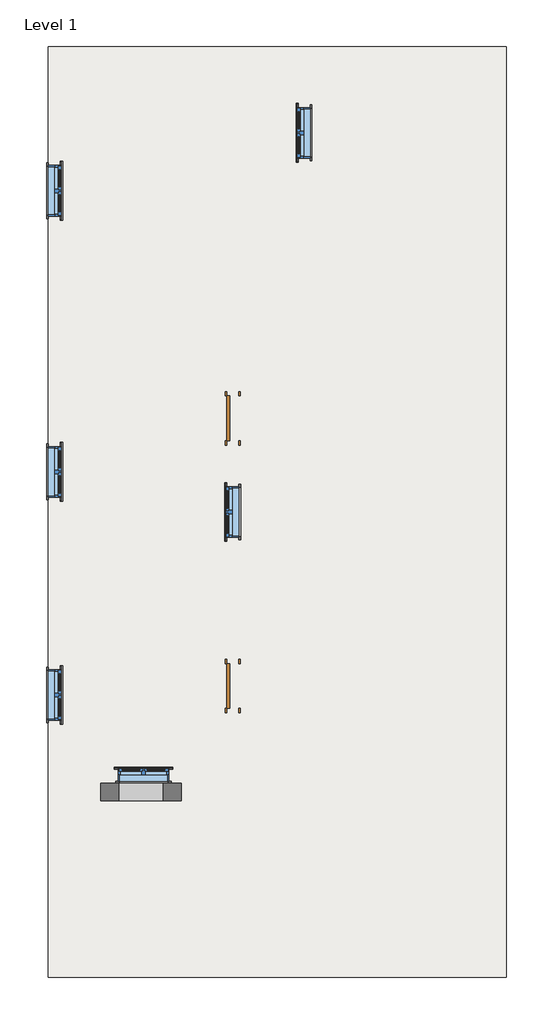
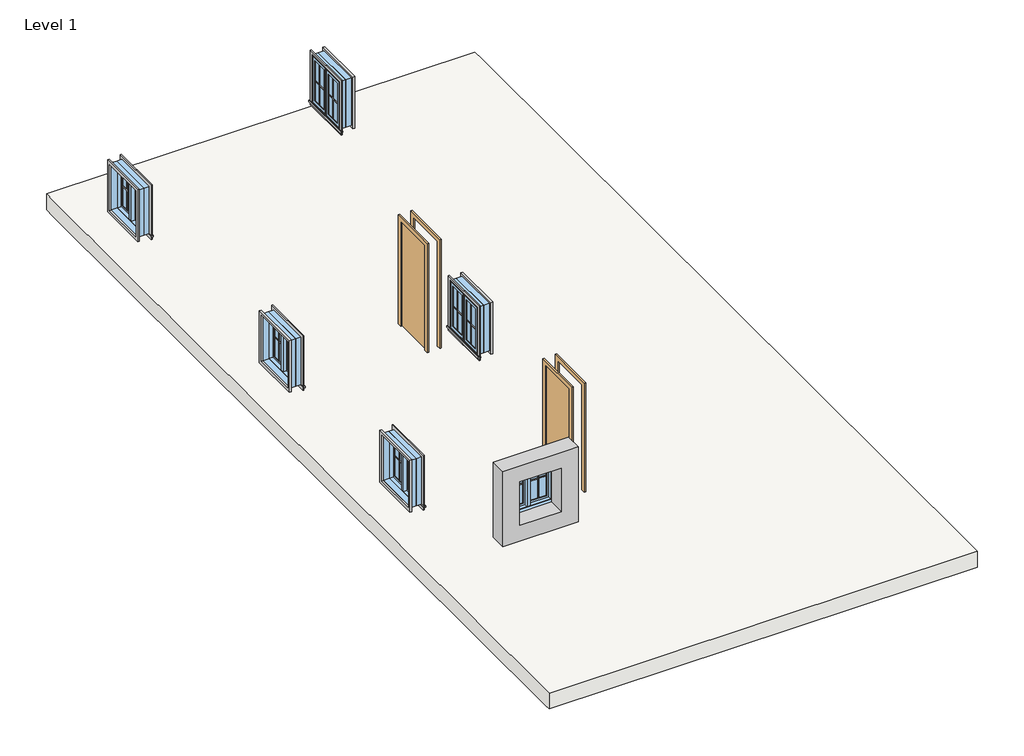
# One storey: 24 proxies, 6 windows, 2 doors, 1 air terminal, 1 slab.
"""IFC4 building model written with IfcOpenShell, lengths in millimetres."""

from ifc_helpers import new_model, si_unit, origin, place, context, project, spatial, faceted_brep, transform, mapped, element, save
from components import air_terminals_1_air_terminals_1_01c5ecaf, muntin_pattern_2x2_muntin_pattern_2x2_b3fe6957, muntin_pattern_2x2_muntin_pattern_2x2_3e0ecaf2, trim_window_exterior_flat_with_sill_41619996, trim_window_interior_flat_picture_frame_51c85655, door_fadea3f2, window_c29befe5

model = new_model("IFC4")

# Units and contexts
model_context = context("Model", 3, world=origin())
ifc_project = project(units=[si_unit("LENGTHUNIT", "METRE", prefix="MILLI")], contexts=[model_context])

# Site, building, storey
site = spatial("IfcSite", under=ifc_project)
building = spatial("IfcBuilding", under=site)
storey = spatial("IfcBuildingStorey", under=building, Name="Level 1", Elevation=5486.4)

# Air terminal
placement = place(None, origin())
air_terminals_1_air_terminals_1_shape = air_terminals_1_air_terminals_1_01c5ecaf(model_context)
element("IfcAirTerminal", 1, ObjectType="Air Terminals 1 : Air Terminals 1", at=placement, inside=storey, context=model_context, shape_type="MappedRepresentation", body=[
    mapped(air_terminals_1_air_terminals_1_shape, transform((0.0, 0.0, 0.0), x_axis=(1.0, 0.0, 0.0), y_axis=(0.0, 1.0, 0.0), z_axis=(0.0, 0.0, 1.0))),
])

# Proxies
muntin_pattern_2x2_muntin_pattern_2x2_shape = muntin_pattern_2x2_muntin_pattern_2x2_b3fe6957(model_context)
element("IfcBuildingElementProxy", 2, Name="Muntin Pattern_2x2 : Muntin Pattern_2x2", ObjectType="Muntin Pattern_2x2 : Muntin Pattern_2x2", at=placement, inside=storey, context=model_context, shape_type="MappedRepresentation", body=[
    mapped(muntin_pattern_2x2_muntin_pattern_2x2_shape, transform((-14472.8012549, 3709.9777962, 6470.65), x_axis=(1.0, 0.0, 0.0), y_axis=(0.0, 1.0, 0.0), z_axis=(0.0, 0.0, 1.0))),
])
element("IfcBuildingElementProxy", 3, Name="Muntin Pattern_2x2 : Muntin Pattern_2x2", ObjectType="Muntin Pattern_2x2 : Muntin Pattern_2x2", at=placement, inside=storey, context=model_context, shape_type="MappedRepresentation", body=[
    mapped(muntin_pattern_2x2_muntin_pattern_2x2_shape, transform((-12826.5637549, 7899.3902962, 6470.65), x_axis=(0.0, 1.0, 0.0), y_axis=(-1.0, 0.0, 0.0), z_axis=(0.0, 0.0, 1.0))),
])
element("IfcBuildingElementProxy", 4, Name="Muntin Pattern_2x2 : Muntin Pattern_2x2", ObjectType="Muntin Pattern_2x2 : Muntin Pattern_2x2", at=placement, inside=storey, context=model_context, shape_type="MappedRepresentation", body=[
    mapped(muntin_pattern_2x2_muntin_pattern_2x2_shape, transform((-15690.4137549, 13814.4152962, 6470.65), x_axis=(0.0, -1.0, 0.0), y_axis=(1.0, 0.0, 0.0), z_axis=(0.0, 0.0, 1.0))),
])
element("IfcBuildingElementProxy", 5, Name="Muntin Pattern_2x2 : Muntin Pattern_2x2", ObjectType="Muntin Pattern_2x2 : Muntin Pattern_2x2", at=placement, inside=storey, context=model_context, shape_type="MappedRepresentation", body=[
    mapped(muntin_pattern_2x2_muntin_pattern_2x2_shape, transform((-15690.4137549, 9013.8152962, 6470.65), x_axis=(0.0, -1.0, 0.0), y_axis=(1.0, 0.0, 0.0), z_axis=(0.0, 0.0, 1.0))),
])
element("IfcBuildingElementProxy", 6, Name="Muntin Pattern_2x2 : Muntin Pattern_2x2", ObjectType="Muntin Pattern_2x2 : Muntin Pattern_2x2", at=placement, inside=storey, context=model_context, shape_type="MappedRepresentation", body=[
    mapped(muntin_pattern_2x2_muntin_pattern_2x2_shape, transform((-15690.4137549, 5203.8152962, 6470.65), x_axis=(0.0, -1.0, 0.0), y_axis=(1.0, 0.0, 0.0), z_axis=(0.0, 0.0, 1.0))),
])
element("IfcBuildingElementProxy", 7, Name="Muntin Pattern_2x2 : Muntin Pattern_2x2", ObjectType="Muntin Pattern_2x2 : Muntin Pattern_2x2", at=placement, inside=storey, context=model_context, shape_type="MappedRepresentation", body=[
    mapped(muntin_pattern_2x2_muntin_pattern_2x2_shape, transform((-11607.3637549, 14376.3902962, 6470.65), x_axis=(0.0, 1.0, 0.0), y_axis=(-1.0, 0.0, 0.0), z_axis=(0.0, 0.0, 1.0))),
])
muntin_pattern_2x2_muntin_pattern_2x2_2_shape = muntin_pattern_2x2_muntin_pattern_2x2_3e0ecaf2(model_context)
element("IfcBuildingElementProxy", 8, Name="Muntin Pattern_2x2 : Muntin Pattern_2x2", ObjectType="Muntin Pattern_2x2 : Muntin Pattern_2x2", at=placement, inside=storey, context=model_context, shape_type="MappedRepresentation", body=[
    mapped(muntin_pattern_2x2_muntin_pattern_2x2_2_shape, transform((-14044.1762549, 3709.9777962, 6470.65), x_axis=(-1.0, 0.0, 0.0), y_axis=(0.0, -1.0, 0.0), z_axis=(0.0, 0.0, 1.0))),
])
element("IfcBuildingElementProxy", 9, Name="Muntin Pattern_2x2 : Muntin Pattern_2x2", ObjectType="Muntin Pattern_2x2 : Muntin Pattern_2x2", at=placement, inside=storey, context=model_context, shape_type="MappedRepresentation", body=[
    mapped(muntin_pattern_2x2_muntin_pattern_2x2_2_shape, transform((-12826.5637549, 8328.0152962, 6470.65), x_axis=(0.0, -1.0, 0.0), y_axis=(1.0, 0.0, 0.0), z_axis=(0.0, 0.0, 1.0))),
])
element("IfcBuildingElementProxy", 10, Name="Muntin Pattern_2x2 : Muntin Pattern_2x2", ObjectType="Muntin Pattern_2x2 : Muntin Pattern_2x2", at=placement, inside=storey, context=model_context, shape_type="MappedRepresentation", body=[
    mapped(muntin_pattern_2x2_muntin_pattern_2x2_2_shape, transform((-15690.4137549, 13385.7902962, 6470.65), x_axis=(0.0, 1.0, 0.0), y_axis=(-1.0, 0.0, 0.0), z_axis=(0.0, 0.0, 1.0))),
])
element("IfcBuildingElementProxy", 11, Name="Muntin Pattern_2x2 : Muntin Pattern_2x2", ObjectType="Muntin Pattern_2x2 : Muntin Pattern_2x2", at=placement, inside=storey, context=model_context, shape_type="MappedRepresentation", body=[
    mapped(muntin_pattern_2x2_muntin_pattern_2x2_2_shape, transform((-15690.4137549, 8585.1902962, 6470.65), x_axis=(0.0, 1.0, 0.0), y_axis=(-1.0, 0.0, 0.0), z_axis=(0.0, 0.0, 1.0))),
])
element("IfcBuildingElementProxy", 12, Name="Muntin Pattern_2x2 : Muntin Pattern_2x2", ObjectType="Muntin Pattern_2x2 : Muntin Pattern_2x2", at=placement, inside=storey, context=model_context, shape_type="MappedRepresentation", body=[
    mapped(muntin_pattern_2x2_muntin_pattern_2x2_2_shape, transform((-15690.4137549, 4775.1902962, 6470.65), x_axis=(0.0, 1.0, 0.0), y_axis=(-1.0, 0.0, 0.0), z_axis=(0.0, 0.0, 1.0))),
])
element("IfcBuildingElementProxy", 13, Name="Muntin Pattern_2x2 : Muntin Pattern_2x2", ObjectType="Muntin Pattern_2x2 : Muntin Pattern_2x2", at=placement, inside=storey, context=model_context, shape_type="MappedRepresentation", body=[
    mapped(muntin_pattern_2x2_muntin_pattern_2x2_2_shape, transform((-11607.3637549, 14805.0152962, 6470.65), x_axis=(0.0, -1.0, 0.0), y_axis=(1.0, 0.0, 0.0), z_axis=(0.0, 0.0, 1.0))),
])
trim_window_exterior_flat_with_sill_shape = trim_window_exterior_flat_with_sill_41619996(model_context)
element("IfcBuildingElementProxy", 14, Name="Trim-Window-Exterior-Flat : with Sill", ObjectType="Trim-Window-Exterior-Flat : with Sill", at=placement, inside=storey, context=model_context, shape_type="MappedRepresentation", body=[
    mapped(trim_window_exterior_flat_with_sill_shape, transform((-14258.4887549, 3719.5027962, 7315.2), x_axis=(-1.0, 0.0, 0.0), y_axis=(0.0, 0.0, 1.0), z_axis=(0.0, 1.0, 0.0))),
])
element("IfcBuildingElementProxy", 15, Name="Trim-Window-Exterior-Flat : with Sill", ObjectType="Trim-Window-Exterior-Flat : with Sill", at=placement, inside=storey, context=model_context, shape_type="MappedRepresentation", body=[
    mapped(trim_window_exterior_flat_with_sill_shape, transform((-12836.0887549, 8113.7027962, 7315.2), x_axis=(0.0, -1.0, 0.0), y_axis=(0.0, 0.0, 1.0), z_axis=(-1.0, 0.0, 0.0))),
])
element("IfcBuildingElementProxy", 16, Name="Trim-Window-Exterior-Flat : with Sill", ObjectType="Trim-Window-Exterior-Flat : with Sill", at=placement, inside=storey, context=model_context, shape_type="MappedRepresentation", body=[
    mapped(trim_window_exterior_flat_with_sill_shape, transform((-15680.8887549, 13600.1027962, 7315.2), x_axis=(0.0, 1.0, 0.0), y_axis=(0.0, 0.0, 1.0), z_axis=(1.0, 0.0, 0.0))),
])
element("IfcBuildingElementProxy", 17, Name="Trim-Window-Exterior-Flat : with Sill", ObjectType="Trim-Window-Exterior-Flat : with Sill", at=placement, inside=storey, context=model_context, shape_type="MappedRepresentation", body=[
    mapped(trim_window_exterior_flat_with_sill_shape, transform((-15680.8887549, 8799.5027962, 7315.2), x_axis=(0.0, 1.0, 0.0), y_axis=(0.0, 0.0, 1.0), z_axis=(1.0, 0.0, 0.0))),
])
element("IfcBuildingElementProxy", 18, Name="Trim-Window-Exterior-Flat : with Sill", ObjectType="Trim-Window-Exterior-Flat : with Sill", at=placement, inside=storey, context=model_context, shape_type="MappedRepresentation", body=[
    mapped(trim_window_exterior_flat_with_sill_shape, transform((-15680.8887549, 4989.5027962, 7315.2), x_axis=(0.0, 1.0, 0.0), y_axis=(0.0, 0.0, 1.0), z_axis=(1.0, 0.0, 0.0))),
])
element("IfcBuildingElementProxy", 19, Name="Trim-Window-Exterior-Flat : with Sill", ObjectType="Trim-Window-Exterior-Flat : with Sill", at=placement, inside=storey, context=model_context, shape_type="MappedRepresentation", body=[
    mapped(trim_window_exterior_flat_with_sill_shape, transform((-11616.8887549, 14590.7027962, 7315.2), x_axis=(0.0, -1.0, 0.0), y_axis=(0.0, 0.0, 1.0), z_axis=(-1.0, 0.0, 0.0))),
])
trim_window_interior_flat_picture_frame_shape = trim_window_interior_flat_picture_frame_51c85655(model_context)
element("IfcBuildingElementProxy", 20, Name="Trim-Window-Interior-Flat : Picture Frame", ObjectType="Trim-Window-Interior-Flat : Picture Frame", at=placement, inside=storey, context=model_context, shape_type="MappedRepresentation", body=[
    mapped(trim_window_interior_flat_picture_frame_shape, transform((-14258.4887549, 3516.3027962, 7315.2), x_axis=(1.0, 0.0, 0.0), y_axis=(0.0, 0.0, 1.0), z_axis=(0.0, -1.0, 0.0))),
])
element("IfcBuildingElementProxy", 21, Name="Trim-Window-Interior-Flat : Picture Frame", ObjectType="Trim-Window-Interior-Flat : Picture Frame", at=placement, inside=storey, context=model_context, shape_type="MappedRepresentation", body=[
    mapped(trim_window_interior_flat_picture_frame_shape, transform((-12632.8887549, 8113.7027962, 7315.2), x_axis=(0.0, 1.0, 0.0), y_axis=(0.0, 0.0, 1.0), z_axis=(1.0, 0.0, 0.0))),
])
element("IfcBuildingElementProxy", 22, Name="Trim-Window-Interior-Flat : Picture Frame", ObjectType="Trim-Window-Interior-Flat : Picture Frame", at=placement, inside=storey, context=model_context, shape_type="MappedRepresentation", body=[
    mapped(trim_window_interior_flat_picture_frame_shape, transform((-15884.0887549, 13600.1027962, 7315.2), x_axis=(0.0, -1.0, 0.0), y_axis=(0.0, 0.0, 1.0), z_axis=(-1.0, 0.0, 0.0))),
])
element("IfcBuildingElementProxy", 23, Name="Trim-Window-Interior-Flat : Picture Frame", ObjectType="Trim-Window-Interior-Flat : Picture Frame", at=placement, inside=storey, context=model_context, shape_type="MappedRepresentation", body=[
    mapped(trim_window_interior_flat_picture_frame_shape, transform((-15884.0887549, 8799.5027962, 7315.2), x_axis=(0.0, -1.0, 0.0), y_axis=(0.0, 0.0, 1.0), z_axis=(-1.0, 0.0, 0.0))),
])
element("IfcBuildingElementProxy", 24, Name="Trim-Window-Interior-Flat : Picture Frame", ObjectType="Trim-Window-Interior-Flat : Picture Frame", at=placement, inside=storey, context=model_context, shape_type="MappedRepresentation", body=[
    mapped(trim_window_interior_flat_picture_frame_shape, transform((-15884.0887549, 4989.5027962, 7315.2), x_axis=(0.0, -1.0, 0.0), y_axis=(0.0, 0.0, 1.0), z_axis=(-1.0, 0.0, 0.0))),
])
element("IfcBuildingElementProxy", 25, Name="Trim-Window-Interior-Flat : Picture Frame", ObjectType="Trim-Window-Interior-Flat : Picture Frame", at=placement, inside=storey, context=model_context, shape_type="MappedRepresentation", body=[
    mapped(trim_window_interior_flat_picture_frame_shape, transform((-11413.6887549, 14590.7027962, 7315.2), x_axis=(0.0, 1.0, 0.0), y_axis=(0.0, 0.0, 1.0), z_axis=(1.0, 0.0, 0.0))),
])

# Doors
door_shape = door_fadea3f2(model_context)
element("IfcDoor", 26, ObjectType="Single-Flush : 30\" x 80\"", at=placement, inside=storey, context=model_context, shape_type="MappedRepresentation", body=[
    mapped(door_shape, transform((-12734.4887549, 9713.9027962, 5486.4), x_axis=(0.0, 1.0, 0.0), y_axis=(-1.0, 0.0, 0.0), z_axis=(0.0, 0.0, 1.0))),
])
element("IfcDoor", 27, ObjectType="Single-Flush : 30\" x 80\"", at=placement, inside=storey, context=model_context, shape_type="MappedRepresentation", body=[
    mapped(door_shape, transform((-12734.4887549, 5141.9027962, 5486.4), x_axis=(0.0, 1.0, 0.0), y_axis=(-1.0, 0.0, 0.0), z_axis=(0.0, 0.0, 1.0))),
])

# Slab
element("IfcSlab", 28, ObjectType="Generic - 12\"", at=placement, inside=storey, context=model_context, shape_type="Brep", body=[
    faceted_brep([(-8060.8887549, 16063.9027962, 5181.6), (-8060.8887549, 15860.7027962, 5181.6), (-8060.8887549, 265.1027962, 5181.6), (-8060.8887549, 163.5027962, 5181.6), (-15884.0887549, 163.5027962, 5181.6), (-15884.0887549, 265.1027962, 5181.6), (-15884.0887549, 15860.7027962, 5181.6), (-15884.0887549, 16063.9027962, 5181.6), (-8060.8887549, 16063.9027962, 5486.4), (-15884.0887549, 16063.9027962, 5486.4), (-15884.0887549, 15860.7027962, 5486.4), (-15884.0887549, 265.1027962, 5486.4), (-15884.0887549, 163.5027962, 5486.4), (-8060.8887549, 163.5027962, 5486.4), (-8060.8887549, 265.1027962, 5486.4), (-8060.8887549, 15860.7027962, 5486.4)], [[[0, 1, 2, 3, 4, 5, 6, 7]], [[8, 9, 10, 11, 12, 13, 14, 15]], [[3, 2, 1, 0, 8, 15, 14, 13]], [[4, 3, 13, 12]], [[7, 6, 5, 4, 12, 11, 10, 9]], [[0, 7, 9, 8]]]),
])

# Windows
window_shape = window_c29befe5(model_context)
element("IfcWindow", 29, ObjectType="Window-Casement-Double : 34\" x 36\"", at=placement, inside=storey, context=model_context, shape_type="MappedRepresentation", body=[
    mapped(window_shape, transform((-14258.4887549, 3617.9027962, 5486.4), x_axis=(1.0, 0.0, 0.0), y_axis=(0.0, 1.0, 0.0), z_axis=(0.0, 0.0, 1.0))),
])
element("IfcWindow", 30, ObjectType="Window-Casement-Double : 34\" x 36\"", at=placement, inside=storey, context=model_context, shape_type="MappedRepresentation", body=[
    mapped(window_shape, transform((-12734.4887549, 8113.7027962, 5486.4), x_axis=(0.0, 1.0, 0.0), y_axis=(-1.0, 0.0, 0.0), z_axis=(0.0, 0.0, 1.0))),
])
element("IfcWindow", 31, ObjectType="Window-Casement-Double : 34\" x 36\"", at=placement, inside=storey, context=model_context, shape_type="MappedRepresentation", body=[
    mapped(window_shape, transform((-15782.4887549, 13600.1027962, 5486.4), x_axis=(0.0, -1.0, 0.0), y_axis=(1.0, 0.0, 0.0), z_axis=(0.0, 0.0, 1.0))),
])
element("IfcWindow", 32, ObjectType="Window-Casement-Double : 34\" x 36\"", at=placement, inside=storey, context=model_context, shape_type="MappedRepresentation", body=[
    mapped(window_shape, transform((-15782.4887549, 8799.5027962, 5486.4), x_axis=(0.0, -1.0, 0.0), y_axis=(1.0, 0.0, 0.0), z_axis=(0.0, 0.0, 1.0))),
])
element("IfcWindow", 33, ObjectType="Window-Casement-Double : 34\" x 36\"", at=placement, inside=storey, context=model_context, shape_type="MappedRepresentation", body=[
    mapped(window_shape, transform((-15782.4887549, 4989.5027962, 5486.4), x_axis=(0.0, -1.0, 0.0), y_axis=(1.0, 0.0, 0.0), z_axis=(0.0, 0.0, 1.0))),
])
element("IfcWindow", 34, ObjectType="Window-Casement-Double : 34\" x 36\"", at=placement, inside=storey, context=model_context, shape_type="MappedRepresentation", body=[
    mapped(window_shape, transform((-11515.2887549, 14590.7027962, 5486.4), x_axis=(0.0, 1.0, 0.0), y_axis=(-1.0, 0.0, 0.0), z_axis=(0.0, 0.0, 1.0))),
])

save(model, "model.ifc")

# Revit data of these elements
# Type "Muntin Pattern_2x2 : Muntin Pattern_2x2"
#   Width [instance default] = 4' - 0"
#   Thickness = 0' - 0 1/2"
#   Height [instance default] = 4' - 0"
#   Distance = 0' - 0 3/4"
#   Interior Material [instance default] = none
#   Exterior Material [instance default] = none
#   Default Elevation = 0
# Type "Trim-Window-Exterior-Flat : with Sill"
#   Trim Width = 0' - 2 1/4"
#   Trim Thickness_Picture Frame = 0' - 1 1/4"
#   Trim Thickness_with Sill = 0' - 0 3/4"
#   Sill Thickness = 0' - 1 1/4"
#   Opening Width [instance default] = 2' - 0"
#   Opening Height [instance default] = 3' - 0"
#   Default Elevation = 4' - 0"
#   Sill = yes
#   Picture Frame = no
#   Trim Material [instance default] = none
# Type "Trim-Window-Interior-Flat : Picture Frame"
#   Trim Thickness_Picture Frame = 0' - 1 1/4"
#   Trim Width = 0' - 2 1/4"
#   Trim Thickness_with Sill = 0' - 0 3/4"
#   Sill Thickness = 0' - 1 1/4"
#   Opening Width [instance default] = 2' - 0"
#   Opening Height [instance default] = 3' - 0"
#   Default Elevation = 4' - 0"
#   Sill = no
#   Picture Frame = yes
#   Trim Material [instance default] = none
# Type "Single-Flush : 30\" x 80\""
#   Type Mark = "5"
#   Construction Type Id = "MDOOR"
#   Assembly Code = "C1020"
#   Analytic Construction = "Metal"
#   Thickness = 0' - 2"
#   Heat Transfer Coefficient (U) = 0.651978 BTU/(h·ft²·°F)
#   Height = 6' - 8"
#   Trim Projection Ext = 0' - 1"
#   Trim Projection Int = 0' - 1"
#   Trim Width = 0' - 3"
#   Width = 2' - 6"
#   Define Thermal Properties by = 1
#   Define Thermal Properties by = 1
#   Door Material = Door - Panel
#   Frame Material = Door - Frame
#   Visual Light Transmittance = 0
#   Solar Heat Gain Coefficient = 0
#   Function = (empty or 0)
#   Wall Closure = (empty or 0)
# Type "Generic - 12\""
#   Assembly Code = "B1010"
#   Function = 0
#   Layers, outside or top first: 1' - 0" no material (function 1)
# Type "Window-Casement-Double : 34\" x 36\""
#   Type Mark = "14"
#   Fire Rating = "0.5h"
#   Assembly Code = "B2020100"
#   Analytic Construction = "Double glazing - domestic"
#   Frame Extension [instance default] = 0' - 0 1/4"
#   Window Inset [instance default] = 0' - 0"
#   Wall Thickness [instance default] = 0' - 6"
#   Interior Wall Closure [instance default] = 0' - 2 1/4"
#   Half Width = 1' - 5"
#   Visual Light Transmittance = 0.81
#   Thermal Resistance (R) = 1.8146 (h·ft²·°F)/BTU
#   Solar Heat Gain Coefficient = 0.76
#   Rough Width = 2' - 10 1/2"
#   Rough Height = 3' - 0 1/2"
#   Height = 3' - 0"
#   Heat Transfer Coefficient (U) = 0.5511 BTU/(h·ft²·°F)
#   Exterior Wall Closure [instance default] = 0' - 1 1/4"
#   Extension Jamb [instance default] = 0' - 2 1/4"
#   Default Sill Height = 3' - 0"
#   Width = 2' - 10"
#   Define Thermal Properties by = 0
#   Muntin Visibility = yes
#   Interior Trim Visibility [instance default] = yes
#   Exterior Trim Visibility [instance default] = yes
#   Extension Jamb Visibility [instance default] = yes
#   Interior Trim Material = Wood - Stained
#   Muntin Pattern = Muntin Pattern_2x2 : Muntin Pattern_2x2
#   Interior Trim = Trim-Window-Interior-Flat : Picture Frame
#   Interior Frame Material = Wood - Stained
#   Glass Panel Material = Glass
#   Exterior Trim Material = Clad - White
#   Exterior Trim = Trim-Window-Exterior-Flat : with Sill
#   Exterior Frame Material = Clad - White
#   Wall Closure = (empty or 0)
# Element 1 (IfcAirTerminal, "Air Terminals 1 : Air Terminals 1")
#   Mark = "1"
#   Phase Created = New Construction
# Elements 2, 3, 4, 5, 6, 7, 8, 9, 10, 11, 12, 13 (IfcBuildingElementProxy, "Muntin Pattern_2x2 : Muntin Pattern_2x2")
#   Width = 0' - 11 5/8"
#   Height = 2' - 6 1/2"
#   Interior Material = Wood - Stained
#   Exterior Material = Clad - White
#   Phase Created = New Construction
#   Materials on its faces: "Clad - White", "Wood - Stained"
# Elements 14, 15, 16, 17, 18, 19 (IfcBuildingElementProxy, "Trim-Window-Exterior-Flat : with Sill")
#   Opening Width = 2' - 10"
#   Opening Height = 3' - 0"
#   Trim Material = Clad - White
#   Phase Created = New Construction
#   Materials on its faces: "Clad - White"
# Elements 20, 21, 22, 23, 24, 25 (IfcBuildingElementProxy, "Trim-Window-Interior-Flat : Picture Frame")
#   Opening Width = 2' - 10"
#   Opening Height = 3' - 0"
#   Trim Material = Wood - Stained
#   Phase Created = New Construction
#   Materials on its faces: "Wood - Stained"
# Elements 26, 27 (IfcDoor, "Single-Flush : 30\" x 80\"")
#   Phase Created = New Construction
#   Materials on its faces: "Door - Frame", "Door - Panel"
# Element 28 (IfcSlab, "Generic - 12\"")
#   Height Offset From Level = 0' - 0"
#   Phase Created = New Construction
#   Materials on its faces: "Default Floor"
# Element 29 (IfcWindow, "Window-Casement-Double : 34\" x 36\"")
#   Mark = "6"
#   Window Inset = 0' - 0"
#   Interior Wall Closure = 0' - 2 1/4"
#   Frame Extension = 0' - 0 1/4"
#   Exterior Wall Closure = 0' - 1 1/4"
#   Interior Trim Visibility = yes
#   Exterior Trim Visibility = yes
#   Phase Created = New Construction
#   Materials on its faces: "Wood - Stained", "Glass", "Clad - White"
# Element 30 (IfcWindow, "Window-Casement-Double : 34\" x 36\"")
#   Mark = "7"
#   Window Inset = 0' - 0"
#   Interior Wall Closure = 0' - 2 1/4"
#   Frame Extension = 0' - 0 1/4"
#   Exterior Wall Closure = 0' - 1 1/4"
#   Interior Trim Visibility = yes
#   Exterior Trim Visibility = yes
#   Phase Created = New Construction
#   Materials on its faces: "Wood - Stained", "Glass", "Clad - White"
# Element 31 (IfcWindow, "Window-Casement-Double : 34\" x 36\"")
#   Mark = "19"
#   Window Inset = 0' - 0"
#   Interior Wall Closure = 0' - 2 1/4"
#   Frame Extension = 0' - 0 1/4"
#   Exterior Wall Closure = 0' - 1 1/4"
#   Interior Trim Visibility = yes
#   Exterior Trim Visibility = yes
#   Phase Created = New Construction
#   Materials on its faces: "Wood - Stained", "Glass", "Clad - White"
# Element 32 (IfcWindow, "Window-Casement-Double : 34\" x 36\"")
#   Mark = "20"
#   Window Inset = 0' - 0"
#   Interior Wall Closure = 0' - 2 1/4"
#   Frame Extension = 0' - 0 1/4"
#   Exterior Wall Closure = 0' - 1 1/4"
#   Interior Trim Visibility = yes
#   Exterior Trim Visibility = yes
#   Phase Created = New Construction
#   Materials on its faces: "Wood - Stained", "Glass", "Clad - White"
# Element 33 (IfcWindow, "Window-Casement-Double : 34\" x 36\"")
#   Mark = "21"
#   Window Inset = 0' - 0"
#   Interior Wall Closure = 0' - 2 1/4"
#   Frame Extension = 0' - 0 1/4"
#   Exterior Wall Closure = 0' - 1 1/4"
#   Interior Trim Visibility = yes
#   Exterior Trim Visibility = yes
#   Phase Created = New Construction
#   Materials on its faces: "Wood - Stained", "Glass", "Clad - White"
# Element 34 (IfcWindow, "Window-Casement-Double : 34\" x 36\"")
#   Mark = "22"
#   Window Inset = 0' - 0"
#   Interior Wall Closure = 0' - 2 1/4"
#   Frame Extension = 0' - 0 1/4"
#   Exterior Wall Closure = 0' - 1 1/4"
#   Interior Trim Visibility = yes
#   Exterior Trim Visibility = yes
#   Phase Created = New Construction
#   Materials on its faces: "Wood - Stained", "Glass", "Clad - White"
# Materials
#   "Door - Panel": class "Wood", colour RGB 210 159 95, transparency 0, Cost = 0
#   "Door - Frame": colour RGB 118 70 51, transparency 0, Cost = 0
#   "Wood - Stained": class "Wood", colour RGB 224 178 126, transparency 0, Cost = 0
#   "Glass": class "Glass", colour RGB 0 128 192, transparency 0.75, Description = "Soda Lime Glass", Cost = 0
#   "Clad - White": class "Wood", colour RGB 242 242 238, transparency 0, Cost = 0
#   "Default Floor": colour RGB 128 128 128, transparency 0, Cost = 0
